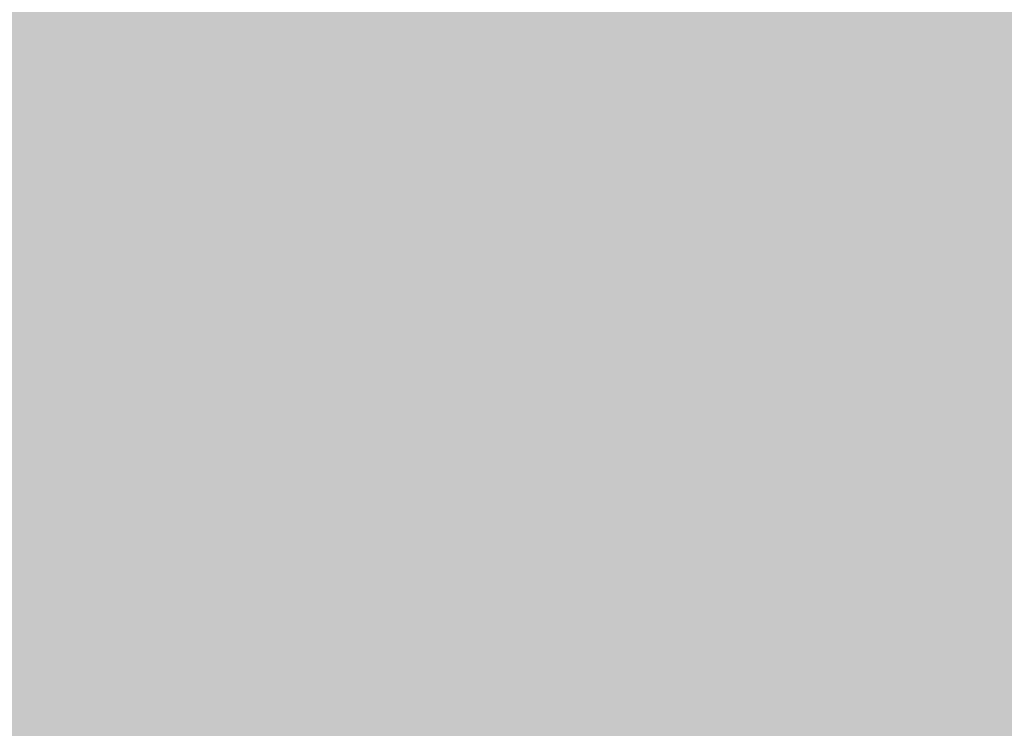
# Model space of a CAD drawing. Units: feet. Extents: x 3168 to 4724, y 827 to 1477.
# Tile 121 of 256: x 3298.685 to 3307.378, y 1087.401 to 1093.654. Entities that reach past the tile are written whole.
import ezdxf

# ---------------------------------------------------------------- set-up
doc = ezdxf.new("R2010")
doc.units = ezdxf.units.FT
doc.layers.add('A-ELEV-PATT', color=8, linetype='Continuous', lineweight=13)

msp = doc.modelspace()

# ---------------------------------------------------------------- hatches: boundary and pattern name
at = {"layer": 'A-ELEV-PATT'}
h = msp.add_hatch(color=256, dxfattribs=at)
h.dxf.hatch_style = 1
edge = h.paths.add_edge_path()
edge.add_ellipse((3552.9058, 979.2201), major_axis=(36.7449, 0), ratio=0.4848485, start_angle=0, end_angle=360)
edge = h.paths.add_edge_path()
edge.add_ellipse((3559.8916, 929.2523), major_axis=(36.7449, 0), ratio=0.4848485, start_angle=0, end_angle=360)
edge = h.paths.add_edge_path()
edge.add_line((3299.3168, 1198.6061), (3479.9167, 1198.6061))
edge.add_line((3479.9167, 1198.6061), (3479.9167, 1209.8686))
edge.add_spline(control_points=[(3479.9167, 1209.8686), (3464.3012, 1209.8686), (3448.6856, 1209.8686), (3410.9491, 1209.8686), (3388.8282, 1209.8686), (3355.6469, 1209.8686), (3344.5864, 1209.8686), (3327.9957, 1209.8686), (3322.4655, 1209.8686), (3314.1702, 1209.8686), (3311.4051, 1209.8686), (3307.2574, 1209.8686), (3305.8748, 1209.8686), (3303.801, 1209.8686), (3303.1097, 1209.8686), (3302.0728, 1209.8686), (3301.7272, 1209.8686), (3301.2087, 1209.8686), (3301.0359, 1209.8686), (3300.7767, 1209.8686), (3300.6903, 1209.8686), (3300.5606, 1209.8686), (3300.5174, 1209.8686), (3300.4526, 1209.8686), (3300.431, 1209.8686), (3300.3986, 1209.8686), (3300.3878, 1209.8686), (3300.3662, 1209.8686), (3300.3457, 1209.8686), (3300.3455, 1209.8686), (3300.3455, 1209.8686), (3300.3433, 1209.8686), (3300.3411, 1209.8686), (3300.3379, 1209.8686), (3300.3368, 1209.8686), (3300.3339, 1209.8686), (3300.3321, 1209.8686), (3300.3255, 1209.8686), (3300.3207, 1209.8686), (3300.3109, 1209.8686), (3300.306, 1209.8686), (3300.2905, 1209.8686), (3300.28, 1209.8686), (3300.2324, 1209.8688), (3300.1953, 1209.869), (3299.9511, 1209.8706), (3299.7448, 1209.8743), (3299.4368, 1209.8833), (3299.3344, 1209.8868), (3299.1811, 1209.8929), (3299.13, 1209.8951), (3298.6522, 1209.9168), (3298.2295, 1209.9457), (3297.6016, 1210.0024), (3297.3934, 1210.0235), (3297.0827, 1210.0583), (3296.9793, 1210.0705), (3296.293, 1210.1549), (3295.7181, 1210.2434), (3294.8687, 1210.3989), (3294.5877, 1210.4545), (3294.1693, 1210.5433), (3294.0304, 1210.5739), (3291.7071, 1211.1012), (3289.6536, 1211.8134), (3285.7763, 1213.564), (3283.9514, 1214.6035), (3280.5122, 1216.9801), (3278.8972, 1218.3176), (3276.3799, 1220.8295), (3275.416, 1221.9177), (3274.0393, 1223.7077), (3273.581, 1224.3495), (3273.1432, 1225.0163)], knot_values=[39.119033, 39.119033, 39.119033, 39.119033, 39.286353, 39.286353, 39.523379, 39.523379, 39.641892, 39.641892, 39.701148, 39.701148, 39.730777, 39.730777, 39.745591, 39.745591, 39.752998, 39.752998, 39.756701, 39.756701, 39.758553, 39.758553, 39.759479, 39.759479, 39.759942, 39.759942, 39.760173, 39.760173, 39.760289, 39.760289, 39.760405, 39.760405, 39.760463, 39.760463, 39.763389, 39.763389, 39.764851, 39.764851, 39.767304, 39.767304, 39.773825, 39.773825, 39.78057, 39.78057, 39.79477, 39.79477, 39.845194, 39.845194, 40.126715, 40.126715, 40.267476, 40.267476, 40.337856, 40.337856, 40.927023, 40.927023, 41.221606, 41.221606, 41.368898, 41.368898, 42.202622, 42.202622, 42.619485, 42.619485, 42.827916, 42.827916, 46.118323, 46.118323, 49.408731, 49.408731, 52.699139, 52.699139, 54.927489, 54.927489, 56.104228, 56.104228, 56.104228, 56.104228], weights=[1, 1, 1, 1, 1, 1, 1, 1, 1, 1, 1, 1, 1, 1, 1, 1, 1, 1, 1, 1, 1, 1, 1, 1, 1, 1, 1, 1, 1, 1, 1, 1, 1, 1, 1, 1, 1, 1, 1, 1, 1, 1, 1, 1, 1, 1, 1, 1, 1, 1, 1, 1, 1, 1, 1, 1, 1, 1, 1, 1, 1, 1, 1, 1, 1, 1, 1, 1, 1, 1, 1, 1, 1, 1], degree=3, periodic=0)
edge.add_line((3273.1432, 1225.0163), (3273.1432, 1099.0163))
edge.add_line((3273.1432, 1099.0163), (3299.3168, 1099.0163))
edge.add_line((3299.3168, 1099.0163), (3299.3168, 1198.6061))
edge = h.paths.add_edge_path()
edge.add_line((3304.7584, 1324.1581), (3479.9167, 1324.1581))
edge.add_line((3479.9167, 1324.1581), (3479.9167, 1335.7146))
edge.add_line((3479.9167, 1335.7146), (3269.1616, 1335.7146))
edge.add_spline(control_points=[(3269.1616, 1335.7146), (3264.0242, 1335.7146), (3258.3641, 1328.9582), (3259.2643, 1323.9003)], knot_values=[0, 0, 0, 0, 15.412191, 15.412191, 15.412191, 15.412191], degree=3, periodic=0)
edge.add_line((3259.2643, 1323.9003), (3265.5168, 1288.7691))
edge.add_line((3265.5168, 1288.7691), (3275.2651, 1261.5456))
edge.add_line((3275.2651, 1261.5456), (3304.7584, 1261.5456))
edge.add_line((3304.7584, 1261.5456), (3304.7584, 1324.1581))
h = msp.add_hatch(color=256, dxfattribs=at)
h.dxf.hatch_style = 1
h.paths.add_polyline_path([(3384.5252, 1099.0163), (3335.0292, 1099.0163), (3299.3168, 1099.0163), (3273.1432, 1099.0163), (3217.5654, 1099.0163), (3168.0693, 827.1163), (3335.0292, 827.1163)])

doc.saveas('drawing.dxf')
